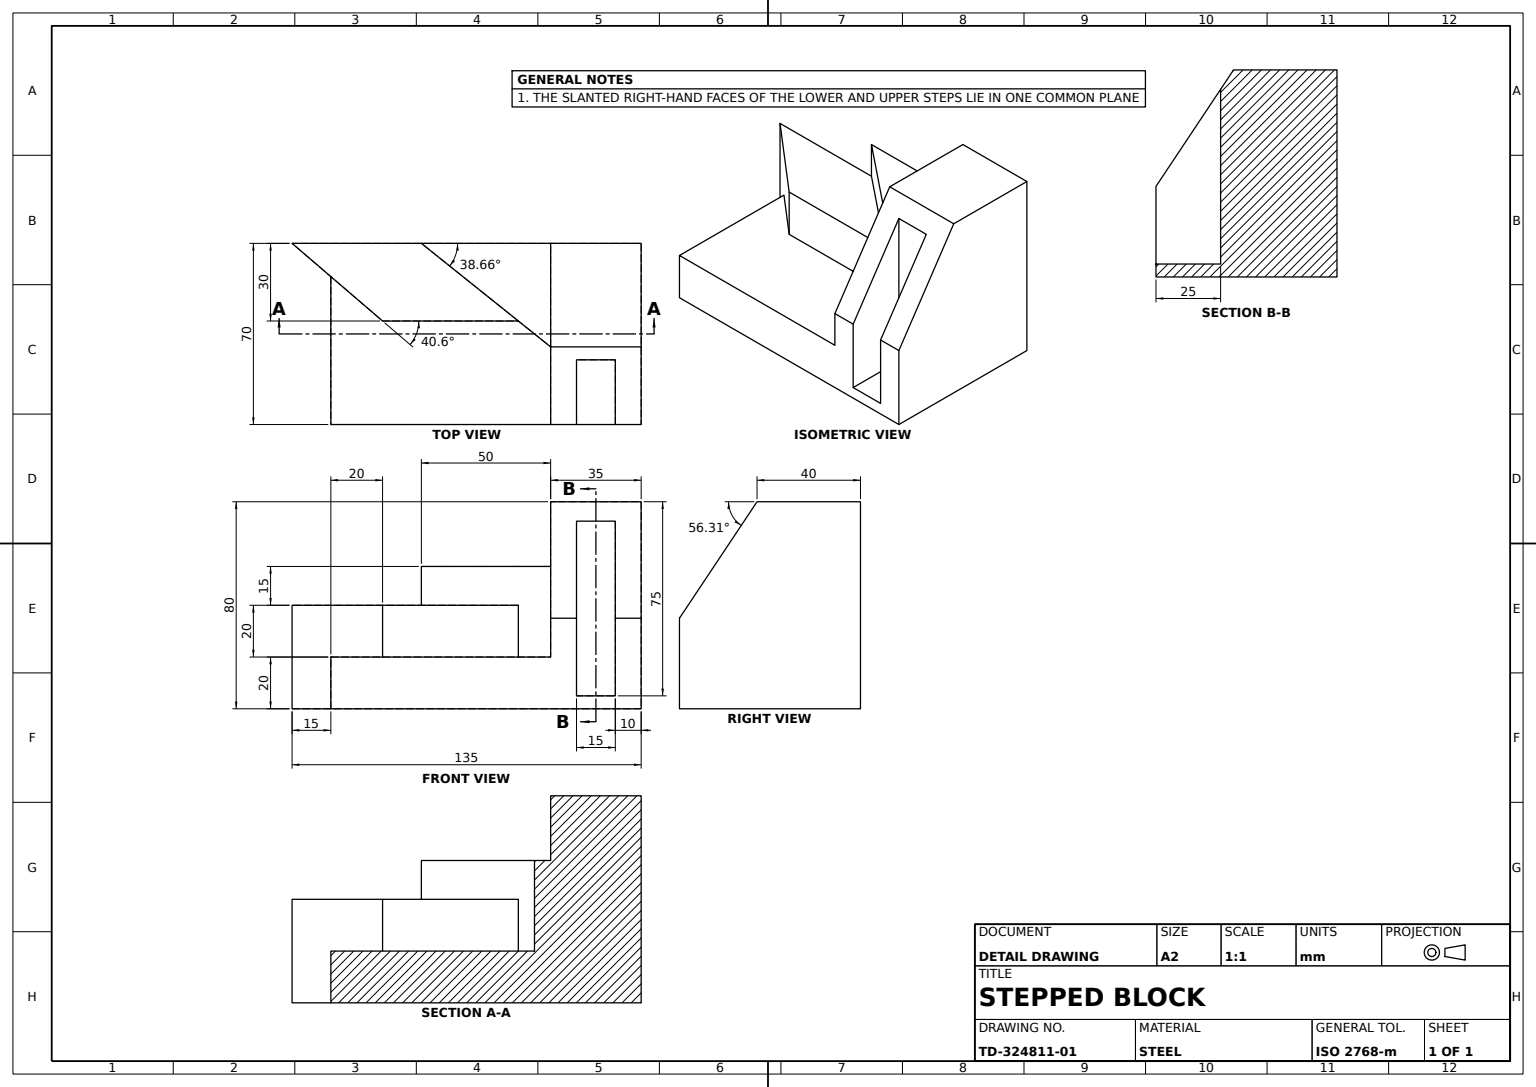
SolidWorks part; units mm, degrees
material "Plain Carbon Steel"
ref_plane "Front Plane" through (0, 0, 0) normal (0, 0, 1) x (1, 0, 0)
ref_plane "Top Plane" through (0, 0, 0) normal (0, 1, 0) x (1, 0, 0)
ref_plane "Right Plane" through (0, 0, 0) normal (1, 0, 0) x (0, 0, -1)
sketch "Base Plate Sketch" plane through (0, 0, 0) normal (0, 1, 0) x (1, 0, 0)
  line L1 (-35, -67.5) -> (35, -67.5)
  line L2 (-35, -67.5) -> (-35, 67.5)
  line L3 (-35, 67.5) -> (35, 67.5)
  line L4 (35, -67.5) -> (35, 67.5)
  line L5 (-35, -67.5) -> (35, 67.5) construction
  line L6 (-35, 67.5) -> (35, -67.5) construction
  point P0 (0, 0)
  dimension "D1" = 135
  dimension "D2" = 70
extrude "Base Plate" add sketch "Base Plate Sketch" along normal blind 20
sketch "Tower Profile Sketch" plane through (0, 0, -67.5) normal (0, 0, -1) x (-1, 0, 0)
  line L0 (35, 0) -> (35, 80)
  line L1 (35, 80) -> (-5, 80)
  line L2 (35, 0) -> (-35, 0)
  line L3 (-35, 0) -> (-35, 35)
  line L4 (-35, 35) -> (-5, 80)
  dimension "D1" = 35
  dimension "D2" = 80
  dimension "D3" = 40
extrude "Tower" add sketch "Tower Profile Sketch" against normal blind 35
sketch "Tower Window Sketch" plane through (0, 80, 0) normal (0, 1, 0) x (1, 0, 0)
  line L0 (35, 32.5) -> (35, 67.5) construction
  line L1 (35, 57.5) -> (10, 57.5)
  line L2 (35, 57.5) -> (35, 42.5)
  line L3 (35, 42.5) -> (10, 42.5)
  line L4 (10, 57.5) -> (10, 42.5)
  line L5 (5, 67.5) -> (35, 67.5) construction
  dimension "D1" = 25
  dimension "D2" = 15
  dimension "D3" = 10
extrude "Tower Window" cut sketch "Tower Window Sketch" against normal blind 75
sketch "Upper Step Sketch" plane through (0, 20, 0) normal (0, 1, 0) x (1, 0, 0)
  line L0 (-35, 32.5) -> (5, 32.5)
  line L1 (-35, 32.5) -> (-35, -17.5)
  line L2 (-35, -17.5) -> (5, 32.5)
  dimension "D1" = 50
extrude "Upper Step" add sketch "Upper Step Sketch" along normal blind 35
sketch "Lower Step Sketch" plane through (0, 20, 0) normal (0, 1, 0) x (1, 0, 0)
  line L0 (-35, -17.5) -> (-35, -67.5)
  line L1 (-35, -67.5) -> (-5, -32.5)
  line L2 (-5, -32.5) -> (-5, 20)
  line L3 (-35, -17.5) -> (5, 32.5) construction
  line L4 (-35, -17.5) -> (-5, 20)
  line L6 (-35, -67.5) -> (35, -67.5) construction
  dimension "D1" = 30
  dimension "D2" = 35
extrude "Lower Step" add sketch "Lower Step Sketch" along normal blind 20
sketch "Step Notch Sketch" plane through (0, 20, 0) normal (0, 1, 0) x (1, 0, 0)
  line L0 (35, -67.5) -> (35, -52.5)
  line L1 (35, -67.5) -> (35, 32.5) construction
  line L2 (35, -52.5) -> (-22.1429, -52.5)
  line L3 (-35, -67.5) -> (-5, -32.5) construction
  line L4 (-22.1429, -52.5) -> (-35, -67.5)
  line L5 (-35, -67.5) -> (35, -67.5)
  dimension "D1" = 15
extrude "Step Notch" cut sketch "Step Notch Sketch" against normal blind 20
